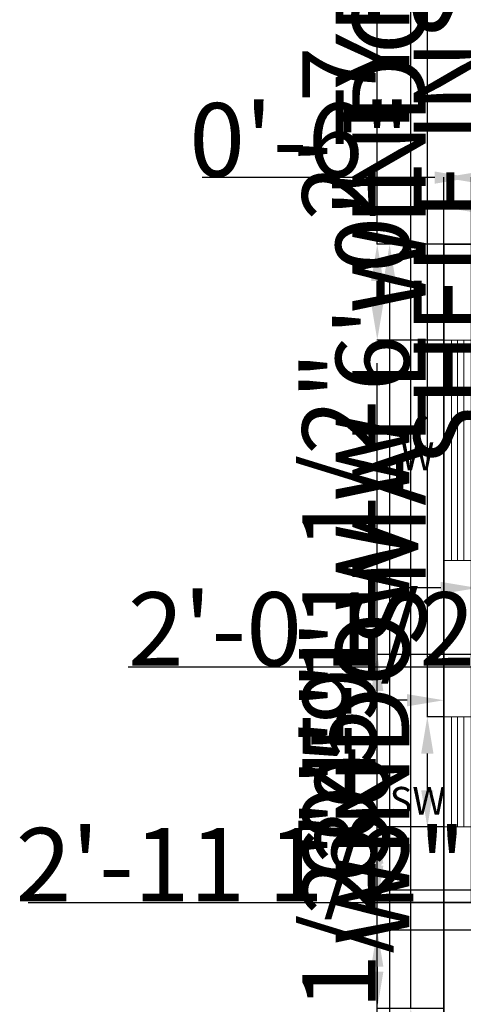
# Model space of a CAD drawing. Units: inches. Extents: x 2236 to 2927, y 1577 to 2452.
# Tile 3 of 9: x 2268 to 2413, y 1836 to 2157. Entities that reach past the tile are written whole.
import ezdxf

# ---------------------------------------------------------------- set-up
doc = ezdxf.new("R2010")
doc.units = ezdxf.units.IN
for name, color, linetype, lineweight in [('A-ANNO-DIMS', 2, 'Continuous', 18), ('A-ANNO-TEXT', 7, 'Continuous', 18), ('Wall', 7, 'Continuous', 35), ('Windows', 162, 'Continuous', 18)]:
    doc.layers.add(name, color=color, linetype=linetype, lineweight=lineweight)
doc.styles.get("Standard").update_dxf_attribs({"font": 'arial.ttf'})
doc.dimstyles.get("Standard").update_dxf_attribs({"dimtxt": 24, "dimasz": 12, "dimexe": 0.18, "dimexo": 0.0625, "dimgap": 0.09, "dimtad": 1, "dimdec": 1, "dimzin": 0, "dimdsep": 46, "dimlunit": 4, "dimtxsty": 'Standard', "dimcen": 0.09, "dimadec": 0, "dimazin": 0, "dimtfac": 1, "dimtdec": 1, "dimtofl": 0, "dimtmove": 0, "dimatfit": 3, "dimfxl": 1, "dimtolj": 1, "dimtzin": 0, "dimarcsym": 0})

# ---------------------------------------------------------------- blocks, each defined once
blk = doc.blocks.new('*D9')
at = {"layer": 'A-ANNO-DIMS', "color": 0, "lineweight": -2, "transparency": 16777216}
for p, q in [((2406.85, 2084.14), (2406.85, 2096.31)), ((2418.85, 2096.13), (2610.85, 2096.13)), ((2622.85, 2084.14), (2622.85, 2096.31))]:
    blk.add_line(p, q, dxfattribs=at)
at = {"layer": 'A-ANNO-DIMS', "color": 0, "transparency": 16777216}
for points in [[(2418.85, 2098.13), (2418.85, 2094.13), (2406.85, 2096.13)], [(2610.85, 2098.13), (2610.85, 2094.13), (2622.85, 2096.13)]]:
    blk.add_solid(points, dxfattribs=at)
at = {"layer": 'Defpoints', "color": 0, "transparency": 16777216}
for p in [(2622.85, 2096.13), (2406.85, 2084.08), (2622.85, 2084.08)]:
    blk.add_point(p, dxfattribs=at)
at = {"layer": 'A-ANNO-DIMS', "color": 0, "transparency": 16777216, "insert": (2514.85, 2108.47), "char_height": 24, "attachment_point": 5}
blk.add_mtext("\\A1;18'", dxfattribs=at)
blk = doc.blocks.new('*D10')
at = {"layer": 'A-ANNO-DIMS', "color": 0, "lineweight": -2, "transparency": 16777216}
for p, q in [((2406.79, 2084.08), (2388.95, 2084.08)), ((2389.13, 2072.08), (2389.13, 1736.08)), ((2406.79, 1724.08), (2388.95, 1724.08))]:
    blk.add_line(p, q, dxfattribs=at)
at = {"layer": 'A-ANNO-DIMS', "color": 0, "transparency": 16777216}
for points in [[(2387.13, 2072.08), (2391.13, 2072.08), (2389.13, 2084.08)], [(2387.13, 1736.08), (2391.13, 1736.08), (2389.13, 1724.08)]]:
    blk.add_solid(points, dxfattribs=at)
at = {"layer": 'Defpoints', "color": 0, "transparency": 16777216}
for p in [(2406.85, 2084.08), (2389.13, 1724.08), (2406.85, 1724.08)]:
    blk.add_point(p, dxfattribs=at)
at = {"layer": 'A-ANNO-DIMS', "color": 0, "transparency": 16777216, "insert": (2376.78, 1904.08), "char_height": 24, "attachment_point": 5, "rotation": 90}
blk.add_mtext("\\A1;30'", dxfattribs=at)
blk = doc.blocks.new('WIN-72IN')
for p, q in [((0, 6.5), (72, 6.5)), ((0, 4.5), (72, 4.5)), ((0, 2.5), (72, 2.5))]:
    blk.add_line(p, q)
blk.add_lwpolyline([(0, 9), (72, 9), (72, 0), (0, 0)], close=True)
blk = doc.blocks.new('WIN-36IN')
for p, q in [((2.5, 0), (2.5, 36)), ((4.5, 0), (4.5, 36)), ((6.5, 0), (6.5, 36))]:
    blk.add_line(p, q)
blk.add_lwpolyline([(0, 0), (0, 36), (9, 36), (9, 0)], close=True)
blk = doc.blocks.new('*D16')
at = {"layer": 'A-ANNO-DIMS', "color": 0, "lineweight": -2, "transparency": 16777216}
for p, q in [((2421.54, 1988.01), (2421.54, 2451.93)), ((2421.05, 1976.01), (2421.72, 1976.01)), ((2421.05, 1972.34), (2421.72, 1972.34)), ((2421.54, 1960.34), (2421.54, 1948.34))]:
    blk.add_line(p, q, dxfattribs=at)
at = {"layer": 'A-ANNO-DIMS', "color": 0, "transparency": 16777216}
for points in [[(2419.54, 1988.01), (2423.54, 1988.01), (2421.54, 1976.01)], [(2419.54, 1960.34), (2423.54, 1960.34), (2421.54, 1972.34)]]:
    blk.add_solid(points, dxfattribs=at)
at = {"layer": 'Defpoints', "color": 0, "transparency": 16777216}
for p in [(2420.99, 1976.01), (2421.54, 1976.01), (2420.99, 1972.34)]:
    blk.add_point(p, dxfattribs=at)
at = {"layer": 'A-ANNO-DIMS', "color": 0, "transparency": 16777216, "insert": (2409.03, 2225.97), "char_height": 24, "attachment_point": 5, "rotation": 90}
blk.add_mtext('\\A1;SHELF INSERT 0\'-3 1/2" TYP.', dxfattribs=at)
blk = doc.blocks.new('*D17')
at = {"layer": 'A-ANNO-DIMS', "color": 0, "lineweight": -2, "transparency": 16777216}
for p, q in [((2405.85, 1971.79), (2393.85, 1971.79)), ((2417.85, 1972.28), (2417.85, 1971.61)), ((2420.99, 1972.28), (2420.99, 1971.61)), ((2432.99, 1971.79), (2591.46, 1971.79))]:
    blk.add_line(p, q, dxfattribs=at)
at = {"layer": 'A-ANNO-DIMS', "color": 0, "transparency": 16777216}
for points in [[(2405.85, 1973.79), (2405.85, 1969.79), (2417.85, 1971.79)], [(2432.99, 1973.79), (2432.99, 1969.79), (2420.99, 1971.79)]]:
    blk.add_solid(points, dxfattribs=at)
at = {"layer": 'Defpoints', "color": 0, "transparency": 16777216}
for p in [(2417.85, 1972.34), (2420.99, 1972.34), (2420.99, 1971.79)]:
    blk.add_point(p, dxfattribs=at)
at = {"layer": 'A-ANNO-DIMS', "color": 0, "transparency": 16777216, "insert": (2518.23, 1984.14), "char_height": 24, "attachment_point": 5}
blk.add_mtext('\\A1;0\'-3" TYP.', dxfattribs=at)
blk = doc.blocks.new('*D18')
at = {"layer": 'A-ANNO-DIMS', "color": 0, "lineweight": -2, "transparency": 16777216}
for p, q in [((2396.05, 1834.44), (2396.05, 2191.28)), ((2406.79, 1834.44), (2395.87, 1834.44)), ((2396.05, 1774.44), (2396.05, 1822.44)), ((2406.79, 1762.44), (2395.87, 1762.44))]:
    blk.add_line(p, q, dxfattribs=at)
at = {"layer": 'A-ANNO-DIMS', "color": 0, "transparency": 16777216}
for points in [[(2394.05, 1822.44), (2398.05, 1822.44), (2396.05, 1834.44)], [(2394.05, 1774.44), (2398.05, 1774.44), (2396.05, 1762.44)]]:
    blk.add_solid(points, dxfattribs=at)
at = {"layer": 'Defpoints', "color": 0, "transparency": 16777216}
for p in [(2396.05, 1834.44), (2406.85, 1834.44), (2406.85, 1762.44)]:
    blk.add_point(p, dxfattribs=at)
at = {"layer": 'A-ANNO-DIMS', "color": 0, "transparency": 16777216, "insert": (2383.54, 2018.86), "char_height": 24, "attachment_point": 5, "rotation": 90}
blk.add_mtext('\\A1;WINDOW W 6\'-0" TYP.', dxfattribs=at)
blk = doc.blocks.new('*D20')
at = {"layer": 'A-ANNO-DIMS', "color": 0, "lineweight": -2, "transparency": 16777216}
for p, q in [((2401.45, 1929.71), (2401.45, 2363.75)), ((2406.79, 1929.71), (2401.27, 1929.71)), ((2401.45, 1905.71), (2401.45, 1917.71)), ((2406.79, 1893.71), (2401.27, 1893.71))]:
    blk.add_line(p, q, dxfattribs=at)
at = {"layer": 'A-ANNO-DIMS', "color": 0, "transparency": 16777216}
for points in [[(2399.45, 1917.71), (2403.45, 1917.71), (2401.45, 1929.71)], [(2399.45, 1905.71), (2403.45, 1905.71), (2401.45, 1893.71)]]:
    blk.add_solid(points, dxfattribs=at)
at = {"layer": 'Defpoints', "color": 0, "transparency": 16777216}
for p in [(2401.45, 1929.71), (2406.85, 1929.71), (2406.85, 1893.71)]:
    blk.add_point(p, dxfattribs=at)
at = {"layer": 'A-ANNO-DIMS', "color": 0, "transparency": 16777216, "insert": (2388.93, 2152.73), "char_height": 24, "attachment_point": 5, "rotation": 90}
blk.add_mtext('\\A1;SMALL WINDOW 3\'-0" TYP.', dxfattribs=at)
blk = doc.blocks.new('*D21')
at = {"layer": 'A-ANNO-DIMS', "color": 0, "lineweight": -2, "transparency": 16777216}
for p, q in [((2394.85, 1935.11), (2382.85, 1935.11)), ((2406.85, 1929.77), (2406.85, 1935.29)), ((2415.85, 1929.77), (2415.85, 1935.29)), ((2427.85, 1935.11), (2586.32, 1935.11))]:
    blk.add_line(p, q, dxfattribs=at)
at = {"layer": 'A-ANNO-DIMS', "color": 0, "transparency": 16777216}
for points in [[(2394.85, 1937.11), (2394.85, 1933.11), (2406.85, 1935.11)], [(2427.85, 1937.11), (2427.85, 1933.11), (2415.85, 1935.11)]]:
    blk.add_solid(points, dxfattribs=at)
at = {"layer": 'Defpoints', "color": 0, "transparency": 16777216}
for p in [(2415.85, 1935.11), (2406.85, 1929.71), (2415.85, 1929.71)]:
    blk.add_point(p, dxfattribs=at)
at = {"layer": 'A-ANNO-DIMS', "color": 0, "transparency": 16777216, "insert": (2513.08, 1947.45), "char_height": 24, "attachment_point": 5}
blk.add_mtext('\\A1;0\'-9" TYP.', dxfattribs=at)
blk = doc.blocks.new('*D23')
at = {"layer": 'A-ANNO-DIMS', "color": 0, "lineweight": -2, "transparency": 16777216}
for p, q in [((2518.6, 1950.01), (2518.6, 1945.71)), ((2543.24, 1950.01), (2543.24, 1945.71)), ((2518.6, 1945.89), (2303.79, 1945.89)), ((2531.24, 1945.89), (2530.6, 1945.89))]:
    blk.add_line(p, q, dxfattribs=at)
at = {"layer": 'A-ANNO-DIMS', "color": 0, "transparency": 16777216}
for points in [[(2530.6, 1947.89), (2530.6, 1943.89), (2518.6, 1945.89)], [(2531.24, 1947.89), (2531.24, 1943.89), (2543.24, 1945.89)]]:
    blk.add_solid(points, dxfattribs=at)
at = {"layer": 'Defpoints', "color": 0, "transparency": 16777216}
for p in [(2518.6, 1950.08), (2543.24, 1950.08), (2518.6, 1945.89)]:
    blk.add_point(p, dxfattribs=at)
at = {"layer": 'A-ANNO-DIMS', "color": 0, "transparency": 16777216, "insert": (2405.19, 1958.39), "char_height": 24, "attachment_point": 5}
blk.add_mtext('\\A1;2\'-0 1/2" TYP.', dxfattribs=at)
blk = doc.blocks.new('*D36')
at = {"layer": 'A-ANNO-DIMS', "color": 0, "lineweight": -2, "transparency": 16777216}
for p, q in [((2454.3, 1796.23), (2454.3, 2047.2)), ((2444.91, 1796.23), (2454.48, 1796.23)), ((2454.3, 1745.23), (2454.3, 1784.23)), ((2444.91, 1733.23), (2454.48, 1733.23))]:
    blk.add_line(p, q, dxfattribs=at)
at = {"layer": 'A-ANNO-DIMS', "color": 0, "transparency": 16777216}
for points in [[(2452.3, 1784.23), (2456.3, 1784.23), (2454.3, 1796.23)], [(2452.3, 1745.23), (2456.3, 1745.23), (2454.3, 1733.23)]]:
    blk.add_solid(points, dxfattribs=at)
at = {"layer": 'Defpoints', "color": 0, "transparency": 16777216}
for p in [(2444.85, 1796.23), (2454.3, 1796.23), (2444.85, 1733.23)]:
    blk.add_point(p, dxfattribs=at)
at = {"layer": 'A-ANNO-DIMS', "color": 0, "transparency": 16777216, "insert": (2441.79, 1927.72), "char_height": 24, "attachment_point": 5, "rotation": 90}
blk.add_mtext('\\A1;SINK UNIT 5\'-3"', dxfattribs=at)
blk = doc.blocks.new('*D38')
at = {"layer": 'A-ANNO-DIMS', "color": 0, "lineweight": -2, "transparency": 16777216}
for p, q in [((2466.44, 1860.06), (2466.44, 2154.67)), ((2457.67, 1860.06), (2466.62, 1860.06)), ((2466.44, 1813.15), (2466.44, 1848.06)), ((2457.67, 1801.15), (2466.62, 1801.15))]:
    blk.add_line(p, q, dxfattribs=at)
at = {"layer": 'A-ANNO-DIMS', "color": 0, "transparency": 16777216}
for points in [[(2464.44, 1848.06), (2468.44, 1848.06), (2466.44, 1860.06)], [(2464.44, 1813.15), (2468.44, 1813.15), (2466.44, 1801.15)]]:
    blk.add_solid(points, dxfattribs=at)
at = {"layer": 'Defpoints', "color": 0, "transparency": 16777216}
for p in [(2457.61, 1860.06), (2466.44, 1860.06), (2457.61, 1801.15)]:
    blk.add_point(p, dxfattribs=at)
at = {"layer": 'A-ANNO-DIMS', "color": 0, "transparency": 16777216, "insert": (2453.94, 2013.36), "char_height": 24, "attachment_point": 5, "rotation": 90}
blk.add_mtext('\\A1;DINING SET 4\'-11"', dxfattribs=at)
blk = doc.blocks.new('*D39')
at = {"layer": 'A-ANNO-DIMS', "color": 0, "lineweight": -2, "transparency": 16777216}
for p, q in [((2422.01, 1868.89), (2271.05, 1868.89)), ((2422.01, 1860.12), (2422.01, 1869.07)), ((2445.61, 1868.89), (2434.01, 1868.89)), ((2457.61, 1860.12), (2457.61, 1869.07))]:
    blk.add_line(p, q, dxfattribs=at)
at = {"layer": 'A-ANNO-DIMS', "color": 0, "transparency": 16777216}
for points in [[(2434.01, 1870.89), (2434.01, 1866.89), (2422.01, 1868.89)], [(2445.61, 1870.89), (2445.61, 1866.89), (2457.61, 1868.89)]]:
    blk.add_solid(points, dxfattribs=at)
at = {"layer": 'Defpoints', "color": 0, "transparency": 16777216}
for p in [(2422.01, 1868.89), (2422.01, 1860.06), (2457.61, 1860.06)]:
    blk.add_point(p, dxfattribs=at)
at = {"layer": 'A-ANNO-DIMS', "color": 0, "transparency": 16777216, "insert": (2340.53, 1881.39), "char_height": 24, "attachment_point": 5}
blk.add_mtext('\\A1;2\'-11 1/2"', dxfattribs=at)
blk = doc.blocks.new('*D40')
at = {"layer": 'A-ANNO-DIMS', "color": 0, "lineweight": -2, "transparency": 16777216}
for p, q in [((2406.85, 2084.14), (2406.85, 2106.01)), ((2418.85, 2105.83), (2433.85, 2105.83)), ((2445.85, 2084.14), (2445.85, 2106.01)), ((2445.85, 2105.83), (2521.81, 2105.83))]:
    blk.add_line(p, q, dxfattribs=at)
at = {"layer": 'A-ANNO-DIMS', "color": 0, "transparency": 16777216}
for points in [[(2418.85, 2107.83), (2418.85, 2103.83), (2406.85, 2105.83)], [(2433.85, 2107.83), (2433.85, 2103.83), (2445.85, 2105.83)]]:
    blk.add_solid(points, dxfattribs=at)
at = {"layer": 'Defpoints', "color": 0, "transparency": 16777216}
for p in [(2445.85, 2105.83), (2406.85, 2084.08), (2445.85, 2084.08)]:
    blk.add_point(p, dxfattribs=at)
at = {"layer": 'A-ANNO-DIMS', "color": 0, "transparency": 16777216, "insert": (2489.83, 2118.18), "char_height": 24, "attachment_point": 5}
blk.add_mtext('\\A1;3\'-3"', dxfattribs=at)
blk = doc.blocks.new('*D42')
at = {"layer": 'A-ANNO-DIMS', "color": 0, "lineweight": -2, "transparency": 16777216}
for p, q in [((2385.1, 2084.08), (2385.1, 2216.39)), ((2406.79, 2084.08), (2384.92, 2084.08)), ((2385.1, 2064.78), (2385.1, 2072.08)), ((2406.79, 2052.78), (2384.92, 2052.78))]:
    blk.add_line(p, q, dxfattribs=at)
at = {"layer": 'A-ANNO-DIMS', "color": 0, "transparency": 16777216}
for points in [[(2383.1, 2072.08), (2387.1, 2072.08), (2385.1, 2084.08)], [(2383.1, 2064.78), (2387.1, 2064.78), (2385.1, 2052.78)]]:
    blk.add_solid(points, dxfattribs=at)
at = {"layer": 'Defpoints', "color": 0, "transparency": 16777216}
for p in [(2385.1, 2084.08), (2406.85, 2084.08), (2406.85, 2052.78)]:
    blk.add_point(p, dxfattribs=at)
at = {"layer": 'A-ANNO-DIMS', "color": 0, "transparency": 16777216, "insert": (2372.6, 2156.23), "char_height": 24, "attachment_point": 5, "rotation": 90}
blk.add_mtext('\\A1;2\'-7 1/2"', dxfattribs=at)
blk = doc.blocks.new('*D43')
at = {"layer": 'A-ANNO-DIMS', "color": 0, "lineweight": -2, "transparency": 16777216}
for p, q in [((2385.1, 1893.71), (2385.1, 2045.22)), ((2406.79, 1893.71), (2384.92, 1893.71)), ((2385.1, 1846.44), (2385.1, 1881.71)), ((2406.79, 1834.44), (2384.92, 1834.44))]:
    blk.add_line(p, q, dxfattribs=at)
at = {"layer": 'A-ANNO-DIMS', "color": 0, "transparency": 16777216}
for points in [[(2383.1, 1881.71), (2387.1, 1881.71), (2385.1, 1893.71)], [(2383.1, 1846.44), (2387.1, 1846.44), (2385.1, 1834.44)]]:
    blk.add_solid(points, dxfattribs=at)
at = {"layer": 'Defpoints', "color": 0, "transparency": 16777216}
for p in [(2385.1, 1893.71), (2406.85, 1893.71), (2406.85, 1834.44)]:
    blk.add_point(p, dxfattribs=at)
at = {"layer": 'A-ANNO-DIMS', "color": 0, "transparency": 16777216, "insert": (2372.6, 1975.46), "char_height": 24, "attachment_point": 5, "rotation": 90}
blk.add_mtext('\\A1;4\'-11 1/2"', dxfattribs=at)
blk = doc.blocks.new('*D44')
at = {"layer": 'A-ANNO-DIMS', "color": 0, "lineweight": -2, "transparency": 16777216}
for p, q in [((2385.1, 1762.44), (2385.1, 1894.33)), ((2406.79, 1762.44), (2384.92, 1762.44)), ((2385.1, 1736.08), (2385.1, 1750.44)), ((2406.79, 1724.08), (2384.92, 1724.08))]:
    blk.add_line(p, q, dxfattribs=at)
at = {"layer": 'A-ANNO-DIMS', "color": 0, "transparency": 16777216}
for points in [[(2383.1, 1750.44), (2387.1, 1750.44), (2385.1, 1762.44)], [(2383.1, 1736.08), (2387.1, 1736.08), (2385.1, 1724.08)]]:
    blk.add_solid(points, dxfattribs=at)
at = {"layer": 'Defpoints', "color": 0, "transparency": 16777216}
for p in [(2385.1, 1762.44), (2406.85, 1762.44), (2406.85, 1724.08)]:
    blk.add_point(p, dxfattribs=at)
at = {"layer": 'A-ANNO-DIMS', "color": 0, "transparency": 16777216, "insert": (2372.59, 1834.38), "char_height": 24, "attachment_point": 5, "rotation": 90}
blk.add_mtext('\\A1;3\'-2 1/2"', dxfattribs=at)
blk = doc.blocks.new('*D47')
at = {"layer": 'A-ANNO-DIMS', "color": 0, "lineweight": -2, "transparency": 16777216}
for p, q in [((2415.79, 1950.08), (2384.92, 1950.08)), ((2385.1, 1885.08), (2385.1, 1938.08)), ((2415.79, 1873.08), (2384.92, 1873.08))]:
    blk.add_line(p, q, dxfattribs=at)
at = {"layer": 'A-ANNO-DIMS', "color": 0, "transparency": 16777216}
for points in [[(2383.1, 1938.08), (2387.1, 1938.08), (2385.1, 1950.08)], [(2383.1, 1885.08), (2387.1, 1885.08), (2385.1, 1873.08)]]:
    blk.add_solid(points, dxfattribs=at)
at = {"layer": 'Defpoints', "color": 0, "transparency": 16777216}
for p in [(2385.1, 1950.08), (2415.85, 1950.08), (2415.85, 1873.08)]:
    blk.add_point(p, dxfattribs=at)
at = {"layer": 'A-ANNO-DIMS', "color": 0, "transparency": 16777216, "insert": (2372.75, 1911.58), "char_height": 24, "attachment_point": 5, "rotation": 90}
blk.add_mtext('\\A1;6\'-5"', dxfattribs=at)
blk = doc.blocks.new('*D60')
at = {"layer": 'A-ANNO-DIMS', "color": 0, "lineweight": -2, "transparency": 16777216}
for p, q in [((2385.1, 1881.08), (2385.1, 1957.05)), ((2415.79, 1869.08), (2384.92, 1869.08)), ((2434.57, 1860.06), (2384.92, 1860.06)), ((2385.1, 1848.06), (2385.1, 1836.06))]:
    blk.add_line(p, q, dxfattribs=at)
at = {"layer": 'A-ANNO-DIMS', "color": 0, "transparency": 16777216}
for points in [[(2383.1, 1881.08), (2387.1, 1881.08), (2385.1, 1869.08)], [(2383.1, 1848.06), (2387.1, 1848.06), (2385.1, 1860.06)]]:
    blk.add_solid(points, dxfattribs=at)
at = {"layer": 'Defpoints', "color": 0, "transparency": 16777216}
for p in [(2385.1, 1869.08), (2415.85, 1869.08), (2434.63, 1860.06)]:
    blk.add_point(p, dxfattribs=at)
at = {"layer": 'A-ANNO-DIMS', "color": 0, "transparency": 16777216, "insert": (2372.75, 1925.07), "char_height": 24, "attachment_point": 5, "rotation": 90}
blk.add_mtext('\\A1;0\'-9"', dxfattribs=at)
blk = doc.blocks.new('*D61')
at = {"layer": 'A-ANNO-DIMS', "color": 0, "lineweight": -2, "transparency": 16777216}
for p, q in [((2403.85, 2105.83), (2327.87, 2105.83)), ((2415.85, 1869.14), (2415.85, 2106.01)), ((2422.01, 1844.91), (2422.01, 2106.01)), ((2434.01, 2105.83), (2446.01, 2105.83))]:
    blk.add_line(p, q, dxfattribs=at)
at = {"layer": 'A-ANNO-DIMS', "color": 0, "transparency": 16777216}
for points in [[(2403.85, 2107.83), (2403.85, 2103.83), (2415.85, 2105.83)], [(2434.01, 2107.83), (2434.01, 2103.83), (2422.01, 2105.83)]]:
    blk.add_solid(points, dxfattribs=at)
at = {"layer": 'Defpoints', "color": 0, "transparency": 16777216}
for p in [(2415.85, 2105.83), (2415.85, 1869.08), (2422.01, 1844.84)]:
    blk.add_point(p, dxfattribs=at)
at = {"layer": 'A-ANNO-DIMS', "color": 0, "transparency": 16777216, "insert": (2359.86, 2118.17), "char_height": 24, "attachment_point": 5}
blk.add_mtext('\\A1;0\'-6"', dxfattribs=at)

msp = doc.modelspace()

# ---------------------------------------------------------------- linework, layer by layer
at = {"layer": 'Wall'}
for q in [(2622.85, 2084.08), (2406.85, 1724.08)]:
    msp.add_line((2406.85, 2084.08), q, dxfattribs=at)

# ---------------------------------------------------------------- block references
at = {"layer": 'Windows', "rotation": 90.00000000000261}
msp.add_blockref('WIN-72IN', (2415.85, 1980.78), dxfattribs=at)
at = {"layer": 'Windows'}
msp.add_blockref('WIN-36IN', (2406.85, 1893.71), dxfattribs=at)

# ---------------------------------------------------------------- texts
at = {"layer": 'A-ANNO-TEXT'}
for s, height, p in [('W', 9.12, (2392.82, 2010.24)), ('SW', 9.116, (2389.13, 1897.69))]:
    msp.add_text(s, height=height, dxfattribs=at).set_placement(p)

# ---------------------------------------------------------------- dimensions: what is measured, and where the dimension line sits
at = {"layer": 'A-ANNO-DIMS'}
for base, p1, p2, angle, text, picture, middle in [((2421.54, 1976.01), (2420.99, 1972.34), (2420.99, 1976.01), 90, 'SHELF INSERT <> TYP.', '*D16', (2409.03, 2225.97)), ((2401.45, 1929.71), (2406.85, 1893.71), (2406.85, 1929.71), 90, 'SMALL WINDOW <> TYP.', '*D20', (2388.93, 2152.73)), ((2396.05, 1834.44), (2406.85, 1762.44), (2406.85, 1834.44), 90, 'WINDOW W <> TYP.', '*D18', (2383.54, 2018.86)), ((2466.44, 1860.06), (2457.61, 1801.15), (2457.61, 1860.06), 90, 'DINING SET <>', '*D38', (2453.94, 2013.36)), ((2454.3, 1796.23), (2444.85, 1733.23), (2444.85, 1796.23), 90, 'SINK UNIT <>', '*D36', (2441.79, 1927.72)), ((2518.6, 1945.89), (2543.24, 1950.08), (2518.6, 1950.08), 180, '<> TYP.', '*D23', (2405.19, 1958.39))]:
    dim = msp.add_linear_dim(base=base, p1=p1, p2=p2, angle=angle, text=text, dimstyle='Standard', override={"dimdec": 1, "dimlfac": 1, "dimrnd": 0, "dimzin": 1, "dimdsep": 46, "dimlunit": 4, "dimfrac": 2}, dxfattribs=at)
    dim.commit()
    dim.dimension.update_dxf_attribs({"geometry": picture, "text_midpoint": middle})
for base, p1, p2, angle, override, picture, middle in [((2385.1, 2084.08), (2406.85, 2052.78), (2406.85, 2084.08), 90, {"dimdec": 1, "dimlfac": 1, "dimrnd": 0, "dimzin": 1, "dimdsep": 46, "dimlunit": 4, "dimfrac": 2}, '*D42', (2372.6, 2156.23)), ((2389.13, 1724.08), (2406.85, 2084.08), (2406.85, 1724.08), 90, {"dimclrd": 0, "dimclre": 0, "dimclrt": 0}, '*D10', (2376.78, 1904.08)), ((2385.1, 1893.71), (2406.85, 1834.44), (2406.85, 1893.71), 90, {"dimdec": 1, "dimlfac": 1, "dimrnd": 0, "dimzin": 1, "dimdsep": 46, "dimlunit": 4, "dimfrac": 2}, '*D43', (2372.6, 1975.46)), ((2385.1, 1869.08), (2434.63, 1860.06), (2415.85, 1869.08), 90, {"dimdec": 1, "dimlfac": 1, "dimrnd": 0, "dimzin": 1, "dimdsep": 46, "dimlunit": 4, "dimfrac": 2}, '*D60', (2372.75, 1925.07)), ((2385.1, 1950.08), (2415.85, 1873.08), (2415.85, 1950.08), 90, {"dimdec": 1, "dimlfac": 1, "dimrnd": 0, "dimzin": 1, "dimdsep": 46, "dimlunit": 4, "dimfrac": 2}, '*D47', (2372.75, 1911.58)), ((2422.01, 1868.89), (2457.61, 1860.06), (2422.01, 1860.06), 180, {"dimdec": 1, "dimlfac": 1, "dimrnd": 0, "dimzin": 1, "dimdsep": 46, "dimlunit": 4, "dimfrac": 2}, '*D39', (2340.53, 1881.39)), ((2385.1, 1762.44), (2406.85, 1724.08), (2406.85, 1762.44), 90, {"dimdec": 1, "dimlfac": 1, "dimrnd": 0, "dimzin": 1, "dimdsep": 46, "dimlunit": 4, "dimfrac": 2}, '*D44', (2372.59, 1834.38))]:
    dim = msp.add_linear_dim(base=base, p1=p1, p2=p2, angle=angle, dimstyle='Standard', override=override, dxfattribs=at)
    dim.commit()
    dim.dimension.update_dxf_attribs({"geometry": picture, "text_midpoint": middle})
for base, p1, p2, override, picture, middle in [((2415.85, 2105.83), (2422.01, 1844.84), (2415.85, 1869.08), {"dimdec": 1, "dimlfac": 1, "dimrnd": 0, "dimzin": 1, "dimdsep": 46, "dimlunit": 4, "dimfrac": 2}, '*D61', (2359.86, 2118.17)), ((2445.85, 2105.83), (2406.85, 2084.08), (2445.85, 2084.08), {"dimdec": 1, "dimlfac": 1, "dimrnd": 0, "dimzin": 1, "dimdsep": 46, "dimlunit": 4, "dimfrac": 2}, '*D40', (2489.83, 2118.18)), ((2622.85, 2096.13), (2406.85, 2084.08), (2622.85, 2084.08), {"dimclrd": 0, "dimclre": 0, "dimclrt": 0}, '*D9', (2514.85, 2108.47))]:
    dim = msp.add_linear_dim(base=base, p1=p1, p2=p2, dimstyle='Standard', override=override, dxfattribs=at)
    dim.commit()
    dim.dimension.update_dxf_attribs({"geometry": picture, "text_midpoint": middle})
for base, p1, p2, picture, middle in [((2420.99, 1971.79), (2417.85, 1972.34), (2420.99, 1972.34), '*D17', (2518.23, 1984.14)), ((2415.85, 1935.11), (2406.85, 1929.71), (2415.85, 1929.71), '*D21', (2513.08, 1947.45))]:
    dim = msp.add_linear_dim(base=base, p1=p1, p2=p2, text='<> TYP.', dimstyle='Standard', override={"dimdec": 1, "dimlfac": 1, "dimrnd": 0, "dimzin": 1, "dimdsep": 46, "dimlunit": 4, "dimfrac": 2}, dxfattribs=at)
    dim.commit()
    dim.dimension.update_dxf_attribs({"geometry": picture, "text_midpoint": middle})

doc.saveas('drawing.dxf')
